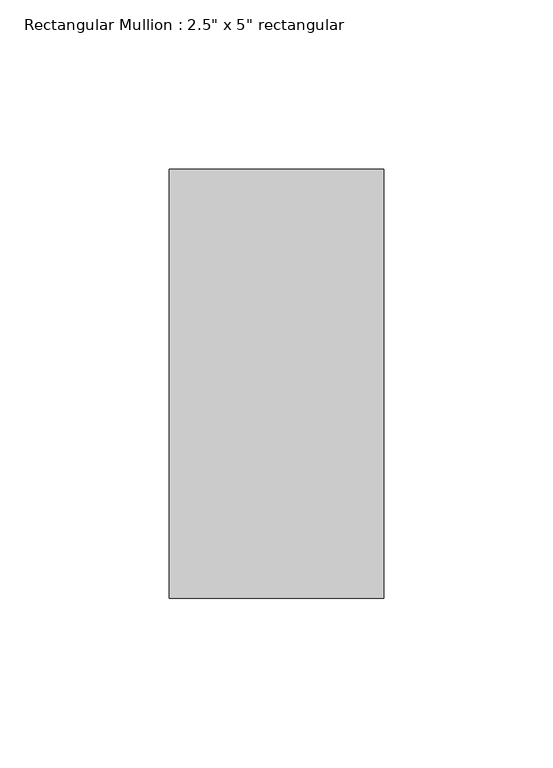
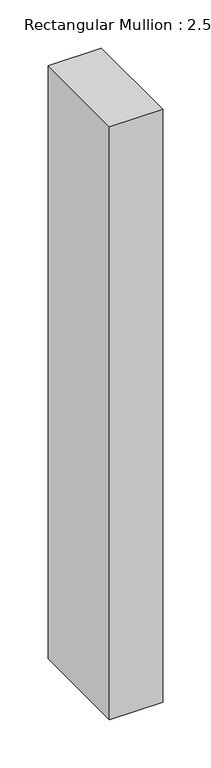
"""IFC4 building model written with IfcOpenShell, lengths in millimetres: member geometry."""

from ifc_helpers import new_model, si_unit, frame, origin, place, context, project, spatial, polyline, outline, extrude, source, transform, mapped, element, save


def member_74f949a7(model_context):
    return source(origin(), model_context, "Body", "SweptSolid", [
        extrude(outline(polyline([(0.0, 63.5), (0.0, -63.5), (-63.5, -63.5), (-63.5, 63.5), (0.0, 63.5)])), frame((0.0, 0.0, -750.616916), z_axis=(0.0, 0.0, 1.0), x_axis=(1.0, 0.0, 0.0)), (0.0, 0.0, 1.0), 750.616916),
    ])


if __name__ == "__main__":
    model = new_model("IFC4")
    model_context = context("Model", 3, world=origin())
    ifc_project = project(units=[si_unit("LENGTHUNIT", "METRE", prefix="MILLI")], contexts=[model_context])
    site = spatial("IfcSite", under=ifc_project)
    building = spatial("IfcBuilding", under=site)
    placement = place(None, origin())
    member_shape = member_74f949a7(model_context)
    element("IfcMember", 1, ObjectType="Rectangular Mullion : 2.5\" x 5\" rectangular", at=placement, inside=building, context=model_context, shape_type="MappedRepresentation", body=[
        mapped(member_shape, transform((0.0, 0.0, 0.0), x_axis=(1.0, 0.0, 0.0), y_axis=(0.0, 1.0, 0.0), z_axis=(0.0, 0.0, 1.0))),
    ])
    save(model, "model.ifc")

# Revit data of these elements
# Type "Rectangular Mullion : 2.5\" x 5\" rectangular"
#   built-in parameter 1007304 = 0.416667 (stored number, unit not read)
#   built-in parameter 1007301 = 0.104167 (stored number, unit not read)
#   built-in parameter 1007300 = 0.104167 (stored number, unit not read)
# Element 1 (IfcMember, "Rectangular Mullion : 2.5\" x 5\" rectangular")
#   Materials on its faces: "Aluminum"
# Materials
#   "Aluminum": class "Metal", colour RGB 247 247 247, transparency 0, Description = "Aluminum 6061", Cost = 0
